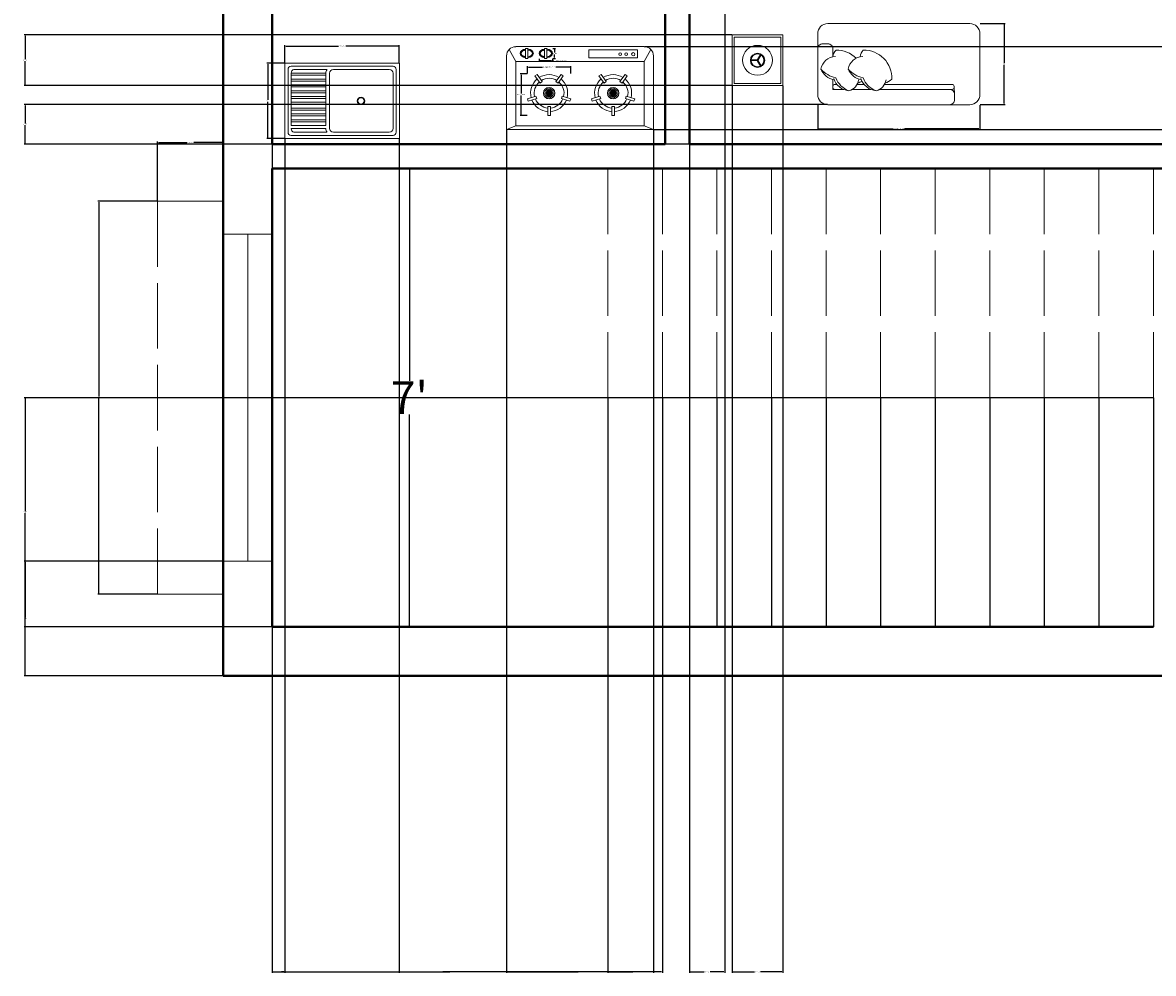
# Model space of a CAD drawing. Units: inches. Extents: x -22 to 362, y -469 to 42.
# Tile 1 of 6: x -22 to 186, y -469 to -295. Entities that reach past the tile are written whole.
import ezdxf

# ---------------------------------------------------------------- set-up
doc = ezdxf.new("R2010")
doc.units = ezdxf.units.IN
doc.header["$MEASUREMENT"] = 0
doc.linetypes.add('ACAD_ISO02W100', pattern=[15, 12, -3])
for name, color, linetype, lineweight in [('A-ANNO-DIMS', 2, 'Continuous', 18), ('A-EQPM', 8, 'Continuous', 18), ('A-FLOR-FIXT', 9, 'Continuous', 20), ('A-FLOR-STRS', 7, 'Continuous', 25), ('A-FLOR-STRS-OVHD', 7, 'ACAD_ISO02W100', 18), ('A-FURN', 8, 'Continuous', 18), ('A-GLAZ', 4, 'Continuous', 20), ('A-ROOF-OVHD', 8, 'ACAD_ISO02W100', 18), ('A-WALL', 7, 'Continuous', 40)]:
    doc.layers.add(name, color=color, linetype=linetype, lineweight=lineweight)
doc.styles.get("Standard").update_dxf_attribs({"font": 'arial.ttf'})
doc.dimstyles.get("Standard").update_dxf_attribs({"dimtxt": 0.18, "dimasz": 0.18, "dimexe": 0.18, "dimexo": 0.0625, "dimgap": 0.09, "dimtad": 0, "dimtih": 1, "dimtoh": 1, "dimdec": 0, "dimzin": 0, "dimdsep": 46, "dimlunit": 3, "dimtxsty": 'Standard', "dimcen": 0.09, "dimadec": 0, "dimazin": 0, "dimtfac": 1, "dimtdec": 0, "dimtofl": 0, "dimtmove": 0, "dimatfit": 3, "dimfxl": 1, "dimtolj": 1, "dimtzin": 0, "dimarcsym": 0})

# ---------------------------------------------------------------- blocks, each defined once
blk = doc.blocks.new('*D1')
at = {"layer": 'A-ANNO-DIMS', "color": 0, "lineweight": -2, "transparency": 16777216}
for p, q in [((49.07, -321.31), (48.96, -321.31)), ((49.14, -321.49), (49.14, -360.22)), ((49.14, -405.13), (49.14, -366.4)), ((49.2, -405.31), (49.32, -405.31))]:
    blk.add_line(p, q, dxfattribs=at)
at = {"layer": 'A-ANNO-DIMS', "color": 0, "transparency": 16777216}
for points in [[(49.11, -321.49), (49.17, -321.49), (49.14, -321.31)], [(49.11, -405.13), (49.17, -405.13), (49.14, -405.31)]]:
    blk.add_solid(points, dxfattribs=at)
at = {"layer": 'Defpoints', "color": 0, "transparency": 16777216}
for p in [(49.14, -321.31), (49.14, -405.31), (49.14, -405.31)]:
    blk.add_point(p, dxfattribs=at)
at = {"layer": 'A-ANNO-DIMS', "color": 0, "transparency": 16777216, "insert": (49.14, -363.31), "char_height": 6, "attachment_point": 5}
blk.add_mtext("\\A1;7'", dxfattribs=at)
blk = doc.blocks.new('DAY BED1')
at = {"color": 0}
blk.add_line((0.3, 0.25), (0.225, 0.255), dxfattribs=at)
blk.add_lwpolyline([(-0.3, 0, -0.414214), (-0.4, 0.1), (-0.4, 0.1, 0.317837), (-0.4, 0.1, -0.414214), (-0.4, 0.1), (-0.4, 0.1, 1.186185), (-0.4, 0.1, -0.414214), (-0.4, 0.1), (-0.4, 1.5, -0.414214), (-0.3, 1.6), (0.3, 1.6, -0.414214), (0.4, 1.5), (0.4, 0.1, -0.414214), (0.3, 0)], format="xyb", close=True, dxfattribs=at)
for points in [[(-0.073, 1.45), (-0.15, 1.45, -0.414214), (-0.2, 1.5), (-0.2, 1.55, -0.414214), (-0.15, 1.6)], [(-0.076, 1.425, -0.356772), (0.05, 1.568, -0.249542), (0.154, 1.438, 9.61688)], [(0.05, 1.568, -0.14773), (0.136, 1.422, -0.213343), (0.262, 1.293, -0.178662)], [(-0.073, 1.45, 0.165541), (-0.139, 1.419, 0.200231), (-0.058, 1.221, 0.121523)], [(0.25, 1.345), (0.25, 1.45), (0.152, 1.45, -0.414214)], [(0.2, 1.412), (0.2, 1.43, -0.414214), (0.22, 1.45), (0.23, 1.45, -0.414214), (0.25, 1.43)], [(0.143, 1.442, -0.306663), (0.262, 1.293, -0.30633), (0.154, 1.196, 0.872847)], [(0.25, 1.43), (0.25, 1.345, -0.414214)], [(-0.076, 1.156, -0.356772), (0.05, 1.299, -0.249542), (0.154, 1.169, 9.61688)], [(0.05, 1.299, -0.14773), (0.136, 1.153, -0.213343), (0.262, 1.024, -0.178662)], [(0.25, 1.262), (0.25, 1.075, -0.414214)], [(-0.073, 1.181, 0.165541), (-0.139, 1.15, 0.425989), (0.148, 0.869, 0.121523), (0.187, 0.936, -7.115464)], [(0.143, 1.173, -0.306663), (0.262, 1.024, -0.30633), (0.154, 0.926, 0.872847)], [(0.168, 1.163, 0.071865), (0.187, 1.205, -7.115464)], [(0.2, 1.142), (0.2, 1.211, -0.414214)], [(0.25, 0.992), (0.25, 0.275, -0.414214), (0.23, 0.255), (0.22, 0.255, -0.414214), (0.2, 0.275), (0.2, 0.942, -0.414214)], [(0.25, 0.377), (0.25, 0.3, 0.414214), (0.3, 0.25), (0.35, 0.25, 0.414214), (0.4, 0.3)]]:
    blk.add_lwpolyline(points, format="xyb", dxfattribs=at)
for points in [[(0.25, 1.075), (0.25, 1.262)], [(0.25, 0.377), (0.25, 0.992)]]:
    blk.add_lwpolyline(points, dxfattribs=at)
blk = doc.blocks.new('М12 540х820')
for p, q in [((0, 540), (-820, 540)), ((-820, 540), (-820, 0)), ((-797.5, 495), (-797.5, 45)), ((-45, 517.5), (-775, 517.5)), ((-347.5, 495), (-748, 495)), ((-301.7, 495), (-64.8, 495)), ((-22.5, 45), (-22.5, 495)), ((0, 0), (0, 540)), ((-775, 468), (-775, 72)), ((-320.5, 468), (-320.5, 72)), ((-293.7, 468), (-293.7, 472.5)), ((-293.7, 468), (-45, 468)), ((-293.7, 446.6), (-45, 446.6)), ((-293.7, 419.6), (-293.7, 446.6)), ((-293.7, 419.6), (-45, 419.6)), ((-45, 469.5), (-45, 468)), ((-45, 419.6), (-45, 446.6)), ((-293.7, 405), (-45, 405)), ((-293.7, 378), (-293.7, 405)), ((-293.7, 378), (-45, 378)), ((-293.7, 336.4), (-293.7, 363.4)), ((-293.7, 363.4), (-45, 363.4)), ((-293.7, 336.4), (-45, 336.4)), ((-45, 378), (-45, 405)), ((-45, 336.4), (-45, 363.4)), ((-293.7, 294.7), (-293.7, 321.7)), ((-293.7, 321.7), (-45, 321.7)), ((-293.7, 294.7), (-45, 294.7)), ((-293.7, 253.1), (-293.7, 280.1)), ((-293.7, 280.1), (-45, 280.1)), ((-293.7, 253.1), (-45, 253.1)), ((-45, 294.7), (-45, 321.7)), ((-45, 253.1), (-45, 280.1)), ((-293.7, 211.5), (-293.7, 238.5)), ((-293.7, 238.5), (-45, 238.5)), ((-293.7, 211.5), (-45, 211.5)), ((-293.7, 169.9), (-293.7, 196.9)), ((-293.7, 196.9), (-45, 196.9)), ((-293.7, 169.9), (-45, 169.9)), ((-45, 211.5), (-45, 238.5)), ((-45, 169.9), (-45, 196.9)), ((-293.7, 128.2), (-293.7, 155.2)), ((-293.7, 155.2), (-45, 155.2)), ((-293.7, 128.2), (-45, 128.2)), ((-293.7, 113.6), (-45, 113.6)), ((-293.7, 86.6), (-293.7, 113.6)), ((-293.7, 86.6), (-45, 86.6)), ((-45, 128.2), (-45, 155.2)), ((-45, 86.6), (-45, 113.6)), ((-820, 0), (0, 0)), ((-775, 22.5), (-45, 22.5)), ((-748, 45), (-347.5, 45)), ((-301.7, 45), (-64.8, 45)), ((-293.7, 72), (-45, 72)), ((-45, 70.5), (-45, 72))]:
    blk.add_line(p, q)
at = {"ltscale": 0.06}
for p, q in [((-820, 0), (-820, 540)), ((-820, 540), (0, 540)), ((0, 540), (0, 536.9)), ((0, 536.9), (0, 0)), ((-293.7, 446.6), (-45, 446.6)), ((-293.7, 405), (-293.7, 446.6)), ((-45, 446.6), (-45, 419.6)), ((-45, 419.6), (-45, 378)), ((-293.7, 363.4), (-293.7, 405)), ((-293.7, 321.7), (-293.7, 363.4)), ((-45, 378), (-45, 336.4)), ((-45, 336.4), (-45, 294.7)), ((-293.7, 280.1), (-293.7, 321.7)), ((-293.7, 238.5), (-293.7, 280.1)), ((-45, 294.7), (-45, 253.1)), ((-45, 253.1), (-45, 211.5)), ((-293.7, 196.9), (-293.7, 238.5)), ((-293.7, 155.2), (-293.7, 196.9)), ((-45, 211.5), (-45, 169.9)), ((-45, 169.9), (-45, 128.2)), ((-293.7, 113.6), (-293.7, 155.2)), ((-293.7, 72), (-293.7, 113.6)), ((-45, 128.2), (-45, 86.6)), ((-45, 86.6), (-45, 72)), ((0, 0), (-820, 0)), ((-45, 72), (-293.7, 72))]:
    blk.add_line(p, q, dxfattribs=at)
at = {"extrusion": (0, 0, -1)}
for centre, major_axis, start_param, end_param in [((-775, 495), (-15.9, 15.9), -0.785398, 0.785398), ((-775, 495), (-15.9, 15.9), -0.785398, 0.785398), ((-748, 468), (-19.1, -19.1), 0.785398, 2.356194), ((-748, 468), (-19.1, -19.1), 0.785398, 2.356194), ((-347.5, 468), (-19.1, 19.1), 0.785398, 2.356194), ((-347.5, 468), (-19.1, 19.1), 0.785398, 2.356194), ((-343.2, 468), (-35, 35), 1.779263, 2.356194), ((-343.2, 468), (-35, 35), 1.779263, 2.356192), ((-72.3, 468.8), (-19.3, 19.3), 1.0328, 2.38382), ((-72.3, 468.8), (-19.3, 19.3), 1.0328, 1.064673), ((-72.3, 468.8), (-19.3, 19.3), 1.064673, 2.328569), ((-45, 495), (-15.9, -15.9), 2.356194, 3.926991), ((-45, 495), (-15.9, -15.9), 2.356194, 3.926991), ((-343.2, 468), (-35, 35), 2.356192, 2.356194), ((-72.3, 468.8), (-19.3, 19.3), 2.328569, 2.38382), ((-545.5, 270), (-19.1, -19.1), 3.926991, 10.210176), ((-545.5, 270), (-19.1, -19.1), 3.926991, 10.210176), ((-545.5, 270), (-15.9, -15.9), 3.926991, 10.210176), ((-545.5, 270), (-15.9, -15.9), 3.926991, 10.210176), ((-775, 45), (-15.9, -15.9), 5.497787, 7.068583), ((-775, 45), (-15.9, -15.9), 5.497787, 7.068583), ((-748, 72), (-19.1, 19.1), 3.926991, 5.497787), ((-748, 72), (-19.1, 19.1), 3.926991, 5.497787), ((-347.5, 72), (-19.1, -19.1), 3.926991, 5.497787), ((-347.5, 72), (-19.1, -19.1), 3.926991, 5.497787), ((-343.2, 72), (-35, -35), 3.926991, 4.503922), ((-343.2, 72), (-35, -35), 3.926991, 4.503922), ((-72.3, 71.2), (-19.3, -19.3), 3.899365, 5.250385), ((-72.3, 71.2), (-19.3, -19.3), 5.218512, 5.250385), ((-72.3, 71.2), (-19.3, -19.3), 3.954617, 5.218512), ((-72.3, 71.2), (-19.3, -19.3), 3.899365, 3.954617), ((-45, 45), (-15.9, 15.9), 2.356194, 3.926991), ((-45, 45), (-15.9, 15.9), 2.356194, 3.926991)]:
    blk.add_ellipse(centre, major_axis=major_axis, ratio=1, start_param=start_param, end_param=end_param, dxfattribs=at)
blk = doc.blocks.new('WIN-60-WALL9')
for p, q in [((0, 9), (60, 9)), ((0, 0), (0, 9)), ((60, 9), (60, 0)), ((0, 4.5), (60, 4.5)), ((60, 0), (0, 0))]:
    blk.add_line(p, q)
blk = doc.blocks.new('WINDOW-SHADE-72')
for p, q in [((12, 72), (0, 72)), ((12, 0), (12, 72)), ((0, 0), (12, 0))]:
    blk.add_line(p, q)
blk = doc.blocks.new('COOKTOP-BURNER')
for p, q in [((-2.59, 3.18), (-2.22, 3.45)), ((-1.63, 1.85), (-2.59, 3.18)), ((-2.22, 3.45), (-1.26, 2.12)), ((-1.26, 2.12), (-1.63, 1.85)), ((1.26, 2.12), (2.22, 3.45)), ((1.63, 1.85), (1.26, 2.12)), ((2.59, 3.18), (1.63, 1.85)), ((2.22, 3.45), (2.59, 3.18)), ((0, 0), (-1.04, 0)), ((0, 0), (-0.99, 0.32)), ((0, 0), (-0.99, -0.32)), ((0, 0), (-0.84, 0.61)), ((0, 0), (-0.84, -0.61)), ((0, 0), (-0.61, 0.84)), ((0, 0), (-0.61, -0.84)), ((0, 0), (-0.32, 0.99)), ((0, 0), (-0.32, -0.99)), ((0, 0), (0, 1.04)), ((0, 0), (0.32, 0.99)), ((0, 0), (0.61, 0.84)), ((0, 0), (0.84, 0.61)), ((0, 0), (0.99, 0.32)), ((0, 0), (1.04, 0)), ((0, 0), (0.99, -0.32)), ((0, 0), (0.84, -0.61)), ((0, 0), (0.61, -0.84)), ((0, 0), (0.32, -0.99)), ((0, 0), (0, -1.04)), ((-3.96, -1.05), (-2.41, -0.54)), ((-3.82, -1.48), (-3.96, -1.05)), ((-2.26, -0.98), (-3.82, -1.48)), ((-2.41, -0.54), (-2.26, -0.98)), ((2.26, -0.98), (2.41, -0.54)), ((3.82, -1.48), (2.26, -0.98)), ((2.41, -0.54), (3.96, -1.05)), ((3.96, -1.05), (3.82, -1.48)), ((-0.23, -2.46), (0.23, -2.46)), ((-0.23, -4.09), (-0.23, -2.46)), ((0.23, -4.09), (-0.23, -4.09)), ((0.23, -2.46), (0.23, -4.09))]:
    blk.add_line(p, q)
blk.add_circle((0, 0), 1.04)
for radius, start, end in [(3.4, 129.8765, 194.1235), (3.4, 57.8765, 122.1235), (2.73, 58.8365, 121.1635), (3.4, 345.8765, 50.1235), (2.73, 130.8365, 193.1635), (2.73, 346.8365, 49.1635), (3.4, 201.8765, 266.1235), (2.73, 202.8365, 265.1635), (2.73, 274.8365, 337.1635), (3.4, 273.8765, 338.1235)]:
    blk.add_arc((0, 0), radius, start, end)
blk = doc.blocks.new('COOKTOP-CONTROL')
for p, q in [((0, 0), (0, 1.86)), ((0, 1.86), (0.44, 1.86)), ((0.44, 0), (0, 0)), ((0.44, 1.86), (0.44, 0))]:
    blk.add_line(p, q)
for major_axis, start_param, end_param in [((1.21, 0), 1.774361, 4.508825), ((-1.21, 0), 1.73081, 4.552375)]:
    blk.add_ellipse((0.24, 0.94), major_axis=major_axis, ratio=0.671641, start_param=start_param, end_param=end_param)
for points, knots in [([(0, 1.56), (-0.06, 1.55), (-0.12, 1.54), (-0.24, 1.51), (-0.31, 1.48), (-0.44, 1.42), (-0.5, 1.39), (-0.59, 1.32), (-0.64, 1.28), (-0.71, 1.2), (-0.73, 1.15), (-0.77, 1.07), (-0.78, 1.03), (-0.8, 0.95), (-0.79, 0.91), (-0.78, 0.83), (-0.76, 0.79), (-0.72, 0.7), (-0.69, 0.66), (-0.61, 0.58), (-0.57, 0.54), (-0.46, 0.47), (-0.4, 0.44), (-0.27, 0.39), (-0.2, 0.36), (-0.09, 0.33), (-0.04, 0.32), (0, 0.32)], [8.079302, 8.079302, 8.079302, 8.079302, 8.245651, 8.245651, 8.463703, 8.463703, 8.681755, 8.681755, 8.899807, 8.899807, 9.117859, 9.117859, 9.33591, 9.33591, 9.553962, 9.553962, 9.772014, 9.772014, 9.990066, 9.990066, 10.208118, 10.208118, 10.426169, 10.426169, 10.644221, 10.644221, 10.770253, 10.770253, 10.770253, 10.770253]), ([(0.44, 0.31), (0.48, 0.32), (0.53, 0.32), (0.64, 0.35), (0.72, 0.37), (0.85, 0.42), (0.91, 0.45), (1.02, 0.52), (1.07, 0.56), (1.15, 0.64), (1.19, 0.68), (1.24, 0.76), (1.26, 0.8), (1.28, 0.87), (1.28, 0.91), (1.28, 0.94), (1.28, 0.98), (1.27, 1.02), (1.25, 1.1), (1.23, 1.15), (1.17, 1.23), (1.13, 1.27), (1.05, 1.35), (0.99, 1.38), (0.88, 1.45), (0.81, 1.48), (0.68, 1.52), (0.6, 1.54), (0.5, 1.56), (0.47, 1.57), (0.44, 1.57)], [4.889299, 4.889299, 4.889299, 4.889299, 5.015191, 5.015191, 5.233243, 5.233243, 5.451295, 5.451295, 5.669347, 5.669347, 5.887399, 5.887399, 6.10545, 6.10545, 6.283185, 6.283185, 6.283185, 6.501237, 6.501237, 6.719289, 6.719289, 6.937341, 6.937341, 7.155392, 7.155392, 7.373444, 7.373444, 7.591496, 7.591496, 7.677072, 7.677072, 7.677072, 7.677072])]:
    blk.add_open_spline(points, degree=3, knots=knots)
blk = doc.blocks.new('*D16')
at = {"layer": 'A-ANNO-DIMS', "color": 0, "lineweight": -2, "transparency": 16777216}
for p, q in [((2.95, -327.31), (-7.97, -327.31)), ((-7.79, -327.49), (-7.79, -363.12)), ((-7.79, -399.13), (-7.79, -363.49)), ((2.95, -399.31), (-7.97, -399.31))]:
    blk.add_line(p, q, dxfattribs=at)
at = {"layer": 'A-ANNO-DIMS', "color": 0, "transparency": 16777216}
for points in [[(-7.82, -327.49), (-7.76, -327.49), (-7.79, -327.31)], [(-7.82, -399.13), (-7.76, -399.13), (-7.79, -399.31)]]:
    blk.add_solid(points, dxfattribs=at)
at = {"layer": 'Defpoints', "color": 0, "transparency": 16777216}
for p in [(3.01, -327.31), (-7.79, -399.31), (3.01, -399.31)]:
    blk.add_point(p, dxfattribs=at)
at = {"layer": 'A-ANNO-DIMS', "color": 0, "transparency": 16777216, "insert": (-7.79, -363.31), "char_height": 0.18, "attachment_point": 5}
blk.add_mtext('\\A1;SHADE 6\'-0" TYP.', dxfattribs=at)
blk = doc.blocks.new('*D17')
at = {"layer": 'A-ANNO-DIMS', "color": 0, "lineweight": -2, "transparency": 16777216}
for p, q in [((3.01, -327.24), (3.01, -316.33)), ((3.19, -316.51), (8.38, -316.51)), ((14.83, -316.51), (9.64, -316.51)), ((15.01, -327.24), (15.01, -316.33))]:
    blk.add_line(p, q, dxfattribs=at)
at = {"layer": 'A-ANNO-DIMS', "color": 0, "transparency": 16777216}
for points in [[(3.19, -316.48), (3.19, -316.54), (3.01, -316.51)], [(14.83, -316.48), (14.83, -316.54), (15.01, -316.51)]]:
    blk.add_solid(points, dxfattribs=at)
at = {"layer": 'Defpoints', "color": 0, "transparency": 16777216}
for p in [(3.01, -316.51), (3.01, -327.31), (15.01, -327.31)]:
    blk.add_point(p, dxfattribs=at)
at = {"layer": 'A-ANNO-DIMS', "color": 0, "transparency": 16777216, "insert": (9.01, -316.51), "char_height": 0.18, "attachment_point": 5}
blk.add_mtext('\\A1;1\'-0" TYP.', dxfattribs=at)
blk = doc.blocks.new('*D24')
at = {"layer": 'A-ANNO-DIMS', "color": 0, "lineweight": -2, "transparency": 16777216}
for p, q in [((70.79, -303.85), (70.79, -302.55)), ((78.72, -303.85), (78.72, -302.55)), ((70.97, -302.73), (73.56, -302.73)), ((78.54, -302.73), (75.96, -302.73))]:
    blk.add_line(p, q, dxfattribs=at)
at = {"layer": 'A-ANNO-DIMS', "color": 0, "transparency": 16777216}
for points in [[(70.97, -302.7), (70.97, -302.76), (70.79, -302.73)], [(78.54, -302.7), (78.54, -302.76), (78.72, -302.73)]]:
    blk.add_solid(points, dxfattribs=at)
at = {"layer": 'Defpoints', "color": 0, "transparency": 16777216}
for p in [(70.79, -303.92), (78.72, -302.73), (78.72, -303.92)]:
    blk.add_point(p, dxfattribs=at)
at = {"layer": 'A-ANNO-DIMS', "color": 0, "transparency": 16777216, "insert": (74.76, -302.73), "char_height": 0.18, "attachment_point": 5}
blk.add_mtext('\\A1;BURNER 0\'-8" TYP.', dxfattribs=at)
blk = doc.blocks.new('*D25')
at = {"layer": 'A-ANNO-DIMS', "color": 0, "lineweight": -2, "transparency": 16777216}
for p, q in [((70.73, -303.92), (69.43, -303.92)), ((69.61, -304.1), (69.61, -307.57)), ((69.61, -311.4), (69.61, -307.93)), ((70.73, -311.58), (69.43, -311.58))]:
    blk.add_line(p, q, dxfattribs=at)
at = {"layer": 'A-ANNO-DIMS', "color": 0, "transparency": 16777216}
for points in [[(69.58, -304.1), (69.64, -304.1), (69.61, -303.92)], [(69.58, -311.4), (69.64, -311.4), (69.61, -311.58)]]:
    blk.add_solid(points, dxfattribs=at)
at = {"layer": 'Defpoints', "color": 0, "transparency": 16777216}
for p in [(69.61, -303.92), (70.79, -303.92), (70.79, -311.58)]:
    blk.add_point(p, dxfattribs=at)
at = {"layer": 'A-ANNO-DIMS', "color": 0, "transparency": 16777216, "insert": (69.61, -307.75), "char_height": 0.18, "attachment_point": 5}
blk.add_mtext('\\A1;0\'-7 1/2" TYP.', dxfattribs=at)
blk = doc.blocks.new('*D26')
at = {"layer": 'A-ANNO-DIMS', "color": 0, "lineweight": -2, "transparency": 16777216}
for p, q in [((72.96, -301.19), (72.96, -301.67)), ((73.14, -301.49), (75.19, -301.49)), ((75.37, -301.19), (75.37, -301.67)), ((75.37, -301.49), (75.55, -301.49))]:
    blk.add_line(p, q, dxfattribs=at)
at = {"layer": 'A-ANNO-DIMS', "color": 0, "transparency": 16777216}
for points in [[(73.14, -301.46), (73.14, -301.52), (72.96, -301.49)], [(75.19, -301.46), (75.19, -301.52), (75.37, -301.49)]]:
    blk.add_solid(points, dxfattribs=at)
at = {"layer": 'Defpoints', "color": 0, "transparency": 16777216}
for p in [(72.96, -301.13), (75.37, -301.13), (75.37, -301.49)]:
    blk.add_point(p, dxfattribs=at)
at = {"layer": 'A-ANNO-DIMS', "color": 0, "transparency": 16777216, "insert": (76.79, -301.49), "char_height": 0.18, "attachment_point": 5}
blk.add_mtext('\\A1;KNOB 0\'-2 1/2" TYP.', dxfattribs=at)
blk = doc.blocks.new('*D27')
at = {"layer": 'A-ANNO-DIMS', "color": 0, "lineweight": -2, "transparency": 16777216}
for p, q in [((75.44, -299.27), (75.92, -299.27)), ((75.74, -299.45), (75.74, -300.02)), ((75.74, -300.95), (75.74, -300.38)), ((75.44, -301.13), (75.92, -301.13))]:
    blk.add_line(p, q, dxfattribs=at)
at = {"layer": 'A-ANNO-DIMS', "color": 0, "transparency": 16777216}
for points in [[(75.71, -299.45), (75.77, -299.45), (75.74, -299.27)], [(75.71, -300.95), (75.77, -300.95), (75.74, -301.13)]]:
    blk.add_solid(points, dxfattribs=at)
at = {"layer": 'Defpoints', "color": 0, "transparency": 16777216}
for p in [(75.37, -299.27), (75.74, -299.27), (75.37, -301.13)]:
    blk.add_point(p, dxfattribs=at)
at = {"layer": 'A-ANNO-DIMS', "color": 0, "transparency": 16777216, "insert": (75.74, -300.2), "char_height": 0.18, "attachment_point": 5}
blk.add_mtext('\\A1;0\'-2" TYP.', dxfattribs=at)
blk = doc.blocks.new('*D28')
at = {"layer": 'A-ANNO-DIMS', "color": 0, "lineweight": -2, "transparency": 16777216}
for p, q in [((123.98, -309.66), (123.98, -314.23)), ((153.72, -309.66), (153.72, -314.23)), ((124.16, -314.05), (137.79, -314.05)), ((153.54, -314.05), (139.91, -314.05))]:
    blk.add_line(p, q, dxfattribs=at)
at = {"layer": 'A-ANNO-DIMS', "color": 0, "transparency": 16777216}
for points in [[(124.16, -314.02), (124.16, -314.08), (123.98, -314.05)], [(153.54, -314.02), (153.54, -314.08), (153.72, -314.05)]]:
    blk.add_solid(points, dxfattribs=at)
at = {"layer": 'Defpoints', "color": 0, "transparency": 16777216}
for p in [(123.98, -309.59), (153.72, -309.59), (123.98, -314.05)]:
    blk.add_point(p, dxfattribs=at)
at = {"layer": 'A-ANNO-DIMS', "color": 0, "transparency": 16777216, "insert": (138.85, -314.05), "char_height": 0.18, "attachment_point": 5}
blk.add_mtext('\\A1;SETTEE 2\'-5 1/2"', dxfattribs=at)
blk = doc.blocks.new('*D29')
at = {"layer": 'A-ANNO-DIMS', "color": 0, "lineweight": -2, "transparency": 16777216}
for p, q in [((153.78, -294.73), (158.36, -294.73)), ((158.18, -294.91), (158.18, -301.98)), ((158.18, -309.41), (158.18, -302.34)), ((153.78, -309.59), (158.36, -309.59))]:
    blk.add_line(p, q, dxfattribs=at)
at = {"layer": 'A-ANNO-DIMS', "color": 0, "transparency": 16777216}
for points in [[(158.15, -294.91), (158.21, -294.91), (158.18, -294.73)], [(158.15, -309.41), (158.21, -309.41), (158.18, -309.59)]]:
    blk.add_solid(points, dxfattribs=at)
at = {"layer": 'Defpoints', "color": 0, "transparency": 16777216}
for p in [(153.72, -294.73), (153.72, -309.59), (158.18, -309.59)]:
    blk.add_point(p, dxfattribs=at)
at = {"layer": 'A-ANNO-DIMS', "color": 0, "transparency": 16777216, "insert": (158.18, -302.16), "char_height": 0.18, "attachment_point": 5}
blk.add_mtext('\\A1;1\'-3"', dxfattribs=at)
blk = doc.blocks.new('*D30')
at = {"layer": 'A-ANNO-DIMS', "color": 0, "lineweight": -2, "transparency": 16777216}
for p, q in [((26.33, -301.93), (26.33, -298.66)), ((26.51, -298.84), (36.16, -298.84)), ((47.12, -298.84), (37.47, -298.84)), ((47.3, -301.93), (47.3, -298.66))]:
    blk.add_line(p, q, dxfattribs=at)
at = {"layer": 'A-ANNO-DIMS', "color": 0, "transparency": 16777216}
for points in [[(26.51, -298.81), (26.51, -298.87), (26.33, -298.84)], [(47.12, -298.81), (47.12, -298.87), (47.3, -298.84)]]:
    blk.add_solid(points, dxfattribs=at)
at = {"layer": 'Defpoints', "color": 0, "transparency": 16777216}
for p in [(26.33, -298.84), (26.33, -301.99), (47.3, -301.99)]:
    blk.add_point(p, dxfattribs=at)
at = {"layer": 'A-ANNO-DIMS', "color": 0, "transparency": 16777216, "insert": (36.81, -298.84), "char_height": 0.18, "attachment_point": 5}
blk.add_mtext('\\A1;SINK 1\'-9"', dxfattribs=at)
blk = doc.blocks.new('*D31')
at = {"layer": 'A-ANNO-DIMS', "color": 0, "lineweight": -2, "transparency": 16777216}
for p, q in [((26.26, -301.99), (23, -301.99)), ((23.18, -302.17), (23.18, -308.72)), ((23.18, -315.62), (23.18, -309.08)), ((26.26, -315.8), (23, -315.8))]:
    blk.add_line(p, q, dxfattribs=at)
at = {"layer": 'A-ANNO-DIMS', "color": 0, "transparency": 16777216}
for points in [[(23.15, -302.17), (23.21, -302.17), (23.18, -301.99)], [(23.15, -315.62), (23.21, -315.62), (23.18, -315.8)]]:
    blk.add_solid(points, dxfattribs=at)
at = {"layer": 'Defpoints', "color": 0, "transparency": 16777216}
for p in [(26.33, -301.99), (23.18, -315.8), (26.33, -315.8)]:
    blk.add_point(p, dxfattribs=at)
at = {"layer": 'A-ANNO-DIMS', "color": 0, "transparency": 16777216, "insert": (23.18, -308.9), "char_height": 0.18, "attachment_point": 5}
blk.add_mtext('\\A1;1\'-2"', dxfattribs=at)
blk = doc.blocks.new('*D37')
at = {"layer": 'A-ANNO-DIMS', "color": 0, "lineweight": -2, "transparency": 16777216}
for p, q in [((14.95, -393.31), (-21.45, -393.31)), ((-21.27, -393.49), (-21.27, -403.62)), ((-21.27, -414.13), (-21.27, -403.99)), ((14.95, -414.31), (-21.45, -414.31))]:
    blk.add_line(p, q, dxfattribs=at)
at = {"layer": 'A-ANNO-DIMS', "color": 0, "transparency": 16777216}
for points in [[(-21.3, -393.49), (-21.24, -393.49), (-21.27, -393.31)], [(-21.3, -414.13), (-21.24, -414.13), (-21.27, -414.31)]]:
    blk.add_solid(points, dxfattribs=at)
at = {"layer": 'Defpoints', "color": 0, "transparency": 16777216}
for p in [(15.01, -393.31), (-21.27, -414.31), (15.01, -414.31)]:
    blk.add_point(p, dxfattribs=at)
at = {"layer": 'A-ANNO-DIMS', "color": 0, "transparency": 16777216, "insert": (-21.27, -403.81), "char_height": 0.18, "attachment_point": 5}
blk.add_mtext('\\A1;1\'-9"', dxfattribs=at)
blk = doc.blocks.new('*D44')
at = {"layer": 'A-ANNO-DIMS', "color": 0, "lineweight": -2, "transparency": 16777216}
for p, q in [((24.01, -405.37), (24.01, -468.77)), ((85.51, -405.37), (85.51, -468.77)), ((24.19, -468.59), (54.22, -468.59)), ((85.33, -468.59), (55.3, -468.59))]:
    blk.add_line(p, q, dxfattribs=at)
at = {"layer": 'A-ANNO-DIMS', "color": 0, "transparency": 16777216}
for points in [[(24.19, -468.56), (24.19, -468.62), (24.01, -468.59)], [(85.33, -468.56), (85.33, -468.62), (85.51, -468.59)]]:
    blk.add_solid(points, dxfattribs=at)
at = {"layer": 'Defpoints', "color": 0, "transparency": 16777216}
for p in [(24.01, -405.31), (85.51, -405.31), (85.51, -468.59)]:
    blk.add_point(p, dxfattribs=at)
at = {"layer": 'A-ANNO-DIMS', "color": 0, "transparency": 16777216, "insert": (54.76, -468.59), "char_height": 0.18, "attachment_point": 5}
blk.add_mtext('\\A1;5\'-1 1/2"', dxfattribs=at)
blk = doc.blocks.new('*D45')
at = {"layer": 'A-ANNO-DIMS', "color": 0, "lineweight": -2, "transparency": 16777216}
for p, q in [((85.51, -405.37), (85.51, -468.77)), ((95.51, -405.37), (95.51, -468.77)), ((85.69, -468.59), (90.11, -468.59)), ((95.33, -468.59), (90.91, -468.59))]:
    blk.add_line(p, q, dxfattribs=at)
at = {"layer": 'A-ANNO-DIMS', "color": 0, "transparency": 16777216}
for points in [[(85.69, -468.56), (85.69, -468.62), (85.51, -468.59)], [(95.33, -468.56), (95.33, -468.62), (95.51, -468.59)]]:
    blk.add_solid(points, dxfattribs=at)
at = {"layer": 'Defpoints', "color": 0, "transparency": 16777216}
for p in [(85.51, -405.31), (95.51, -405.31), (95.51, -468.59)]:
    blk.add_point(p, dxfattribs=at)
at = {"layer": 'A-ANNO-DIMS', "color": 0, "transparency": 16777216, "insert": (90.51, -468.59), "char_height": 0.18, "attachment_point": 5}
blk.add_mtext('\\A1;0\'-10"', dxfattribs=at)
blk = doc.blocks.new('*D46')
at = {"layer": 'A-ANNO-DIMS', "color": 0, "lineweight": -2, "transparency": 16777216}
for p, q in [((85.45, -363.31), (-21.45, -363.31)), ((-21.27, -363.49), (-21.27, -384.12)), ((-21.27, -405.13), (-21.27, -384.49)), ((85.45, -405.31), (-21.45, -405.31))]:
    blk.add_line(p, q, dxfattribs=at)
at = {"layer": 'A-ANNO-DIMS', "color": 0, "transparency": 16777216}
for points in [[(-21.3, -363.49), (-21.24, -363.49), (-21.27, -363.31)], [(-21.3, -405.13), (-21.24, -405.13), (-21.27, -405.31)]]:
    blk.add_solid(points, dxfattribs=at)
at = {"layer": 'Defpoints', "color": 0, "transparency": 16777216}
for p in [(85.51, -363.31), (-21.27, -405.31), (85.51, -405.31)]:
    blk.add_point(p, dxfattribs=at)
at = {"layer": 'A-ANNO-DIMS', "color": 0, "transparency": 16777216, "insert": (-21.27, -384.31), "char_height": 0.18, "attachment_point": 5}
blk.add_mtext('\\A1;3\'-6"', dxfattribs=at)
blk = doc.blocks.new('*D52')
at = {"layer": 'A-ANNO-DIMS', "color": 0, "lineweight": -2, "transparency": 16777216}
for p, q in [((106.94, -292.58), (106.94, -468.77)), ((100.51, -316.87), (100.51, -468.77)), ((100.69, -468.59), (103.19, -468.59)), ((106.76, -468.59), (104.27, -468.59))]:
    blk.add_line(p, q, dxfattribs=at)
at = {"layer": 'A-ANNO-DIMS', "color": 0, "transparency": 16777216}
for points in [[(100.69, -468.56), (100.69, -468.62), (100.51, -468.59)], [(106.76, -468.56), (106.76, -468.62), (106.94, -468.59)]]:
    blk.add_solid(points, dxfattribs=at)
at = {"layer": 'Defpoints', "color": 0, "transparency": 16777216}
for p in [(106.94, -292.52), (100.51, -316.81), (106.94, -468.59)]:
    blk.add_point(p, dxfattribs=at)
at = {"layer": 'A-ANNO-DIMS', "color": 0, "transparency": 16777216, "insert": (103.73, -468.59), "char_height": 0.18, "attachment_point": 5}
blk.add_mtext('\\A1;0\'-6 1/2"', dxfattribs=at)
blk = doc.blocks.new('*D53')
at = {"layer": 'A-ANNO-DIMS', "color": 0, "lineweight": -2, "transparency": 16777216}
for p, q in [((125.78, -309.59), (-21.45, -309.59)), ((-21.27, -309.77), (-21.27, -313.02)), ((-21.27, -316.63), (-21.27, -313.38)), ((100.45, -316.81), (-21.45, -316.81))]:
    blk.add_line(p, q, dxfattribs=at)
at = {"layer": 'A-ANNO-DIMS', "color": 0, "transparency": 16777216}
for points in [[(-21.3, -309.77), (-21.24, -309.77), (-21.27, -309.59)], [(-21.3, -316.63), (-21.24, -316.63), (-21.27, -316.81)]]:
    blk.add_solid(points, dxfattribs=at)
at = {"layer": 'Defpoints', "color": 0, "transparency": 16777216}
for p in [(-21.27, -309.59), (125.84, -309.59), (100.51, -316.81)]:
    blk.add_point(p, dxfattribs=at)
at = {"layer": 'A-ANNO-DIMS', "color": 0, "transparency": 16777216, "insert": (-21.27, -313.2), "char_height": 0.18, "attachment_point": 5}
blk.add_mtext('\\A1;0\'-7"', dxfattribs=at)
blk = doc.blocks.new('*D58')
at = {"layer": 'A-ANNO-DIMS', "color": 0, "lineweight": -2, "transparency": 16777216}
for p, q in [((108.31, -306.17), (108.31, -468.77)), ((117.6, -306.17), (117.6, -468.77)), ((108.49, -468.59), (112.42, -468.59)), ((117.42, -468.59), (113.5, -468.59))]:
    blk.add_line(p, q, dxfattribs=at)
at = {"layer": 'A-ANNO-DIMS', "color": 0, "transparency": 16777216}
for points in [[(108.49, -468.56), (108.49, -468.62), (108.31, -468.59)], [(117.42, -468.56), (117.42, -468.62), (117.6, -468.59)]]:
    blk.add_solid(points, dxfattribs=at)
at = {"layer": 'Defpoints', "color": 0, "transparency": 16777216}
for p in [(108.31, -306.11), (117.6, -306.11), (117.6, -468.59)]:
    blk.add_point(p, dxfattribs=at)
at = {"layer": 'A-ANNO-DIMS', "color": 0, "transparency": 16777216, "insert": (112.96, -468.59), "char_height": 0.18, "attachment_point": 5}
blk.add_mtext('\\A1;0\'-9 1/2"', dxfattribs=at)
blk = doc.blocks.new('*D59')
at = {"layer": 'A-ANNO-DIMS', "color": 0, "lineweight": -2, "transparency": 16777216}
for p, q in [((108.25, -296.82), (-21.45, -296.82)), ((-21.27, -297), (-21.27, -301.28)), ((-21.27, -305.93), (-21.27, -301.64)), ((108.25, -306.11), (-21.45, -306.11))]:
    blk.add_line(p, q, dxfattribs=at)
at = {"layer": 'A-ANNO-DIMS', "color": 0, "transparency": 16777216}
for points in [[(-21.3, -297), (-21.24, -297), (-21.27, -296.82)], [(-21.3, -305.93), (-21.24, -305.93), (-21.27, -306.11)]]:
    blk.add_solid(points, dxfattribs=at)
at = {"layer": 'Defpoints', "color": 0, "transparency": 16777216}
for p in [(108.31, -296.82), (-21.27, -306.11), (108.31, -306.11)]:
    blk.add_point(p, dxfattribs=at)
at = {"layer": 'A-ANNO-DIMS', "color": 0, "transparency": 16777216, "insert": (-21.27, -301.46), "char_height": 0.18, "attachment_point": 5}
blk.add_mtext('\\A1;0\'-9 1/2"', dxfattribs=at)
blk = doc.blocks.new('*D60')
at = {"layer": 'A-ANNO-DIMS', "color": 0, "lineweight": -2, "transparency": 16777216}
for p, q in [((66.94, -314.19), (66.94, -468.77)), ((93.9, -314.19), (93.9, -468.77)), ((67.12, -468.59), (80.09, -468.59)), ((93.72, -468.59), (80.75, -468.59))]:
    blk.add_line(p, q, dxfattribs=at)
at = {"layer": 'A-ANNO-DIMS', "color": 0, "transparency": 16777216}
for points in [[(67.12, -468.56), (67.12, -468.62), (66.94, -468.59)], [(93.72, -468.56), (93.72, -468.62), (93.9, -468.59)]]:
    blk.add_solid(points, dxfattribs=at)
at = {"layer": 'Defpoints', "color": 0, "transparency": 16777216}
for p in [(66.94, -314.13), (93.9, -314.13), (93.9, -468.59)]:
    blk.add_point(p, dxfattribs=at)
at = {"layer": 'A-ANNO-DIMS', "color": 0, "transparency": 16777216, "insert": (80.42, -468.59), "char_height": 0.18, "attachment_point": 5}
blk.add_mtext('\\A1;2\'-3"', dxfattribs=at)
blk = doc.blocks.new('*D61')
at = {"layer": 'A-ANNO-DIMS', "color": 0, "lineweight": -2, "transparency": 16777216}
for p, q in [((92.28, -298.96), (350.97, -298.96)), ((350.79, -299.14), (350.79, -306.36)), ((350.79, -313.95), (350.79, -306.73)), ((93.96, -314.13), (350.97, -314.13))]:
    blk.add_line(p, q, dxfattribs=at)
at = {"layer": 'A-ANNO-DIMS', "color": 0, "transparency": 16777216}
for points in [[(350.76, -299.14), (350.82, -299.14), (350.79, -298.96)], [(350.76, -313.95), (350.82, -313.95), (350.79, -314.13)]]:
    blk.add_solid(points, dxfattribs=at)
at = {"layer": 'Defpoints', "color": 0, "transparency": 16777216}
for p in [(92.21, -298.96), (350.79, -298.96), (93.9, -314.13)]:
    blk.add_point(p, dxfattribs=at)
at = {"layer": 'A-ANNO-DIMS', "color": 0, "transparency": 16777216, "insert": (350.79, -306.55), "char_height": 0.18, "attachment_point": 5}
blk.add_mtext('\\A1;1\'-3"', dxfattribs=at)
blk = doc.blocks.new('*D62')
at = {"layer": 'A-ANNO-DIMS', "color": 0, "lineweight": -2, "transparency": 16777216}
for p, q in [((66.94, -314.19), (66.94, -468.77)), ((47.3, -315.87), (47.3, -468.77)), ((47.48, -468.59), (56.59, -468.59)), ((66.76, -468.59), (57.65, -468.59))]:
    blk.add_line(p, q, dxfattribs=at)
at = {"layer": 'A-ANNO-DIMS', "color": 0, "transparency": 16777216}
for points in [[(47.48, -468.56), (47.48, -468.62), (47.3, -468.59)], [(66.76, -468.56), (66.76, -468.62), (66.94, -468.59)]]:
    blk.add_solid(points, dxfattribs=at)
at = {"layer": 'Defpoints', "color": 0, "transparency": 16777216}
for p in [(66.94, -314.13), (47.3, -315.8), (66.94, -468.59)]:
    blk.add_point(p, dxfattribs=at)
at = {"layer": 'A-ANNO-DIMS', "color": 0, "transparency": 16777216, "insert": (57.12, -468.59), "char_height": 0.18, "attachment_point": 5}
blk.add_mtext('\\A1;1\'-7 1/2"', dxfattribs=at)
blk = doc.blocks.new('*D63')
at = {"layer": 'A-ANNO-DIMS', "color": 0, "lineweight": -2, "transparency": 16777216}
for p, q in [((24.01, -316.87), (24.01, -468.77)), ((26.33, -315.87), (26.33, -468.77)), ((24.19, -468.59), (24.63, -468.59)), ((26.15, -468.59), (25.71, -468.59))]:
    blk.add_line(p, q, dxfattribs=at)
at = {"layer": 'A-ANNO-DIMS', "color": 0, "transparency": 16777216}
for points in [[(24.19, -468.56), (24.19, -468.62), (24.01, -468.59)], [(26.15, -468.56), (26.15, -468.62), (26.33, -468.59)]]:
    blk.add_solid(points, dxfattribs=at)
at = {"layer": 'Defpoints', "color": 0, "transparency": 16777216}
for p in [(24.01, -316.81), (26.33, -315.8), (26.33, -468.59)]:
    blk.add_point(p, dxfattribs=at)
at = {"layer": 'A-ANNO-DIMS', "color": 0, "transparency": 16777216, "insert": (25.17, -468.59), "char_height": 0.18, "attachment_point": 5}
blk.add_mtext('\\A1;0\'-2 1/2"', dxfattribs=at)

msp = doc.modelspace()

# ---------------------------------------------------------------- linework, layer by layer
at = {"layer": 'A-EQPM'}
for p, q in [((68.63, -301.69), (67.44, -299.46)), ((92.21, -298.96), (68.63, -298.96)), ((82.01, -299.54), (90.93, -299.54)), ((82.01, -300.99), (82.01, -299.54)), ((90.93, -299.54), (90.93, -300.99)), ((92.21, -301.69), (93.41, -299.46)), ((66.94, -300.65), (66.94, -314.13)), ((68.63, -301.69), (68.63, -313.49)), ((92.21, -301.69), (68.63, -301.69)), ((90.93, -300.99), (82.01, -300.99)), ((92.21, -313.49), (92.21, -301.69)), ((93.9, -314.13), (93.9, -300.65)), ((68.63, -313.49), (66.94, -314.13)), ((66.94, -314.13), (93.9, -314.13)), ((68.63, -313.49), (92.21, -313.49)), ((92.21, -313.49), (93.9, -314.13))]:
    msp.add_line(p, q, dxfattribs=at)
for centre, radius in [((87.79, -300.34), 0.249), ((88.88, -300.34), 0.249), ((90.18, -300.34), 0.299)]:
    msp.add_circle(centre, radius, dxfattribs=at)
for centre, start, end in [((68.63, -300.65), 90, 180), ((92.21, -300.65), 0, 90)]:
    msp.add_arc(centre, 1.68, start, end, dxfattribs=at)
at = {"layer": 'A-FLOR-STRS'}
for p, q in [((185.51, -363.31), (85.51, -363.31)), ((85.51, -363.31), (85.51, -405.31)), ((95.51, -363.31), (95.51, -405.31)), ((105.51, -363.31), (105.51, -405.31)), ((115.51, -363.31), (115.51, -405.31)), ((125.51, -363.31), (125.51, -405.31)), ((135.51, -363.31), (135.51, -405.31)), ((145.51, -363.31), (145.51, -405.31)), ((155.51, -363.31), (155.51, -405.31)), ((165.51, -363.31), (165.51, -405.31)), ((175.51, -363.31), (175.51, -405.31)), ((185.51, -363.31), (185.51, -405.31))]:
    msp.add_line(p, q, dxfattribs=at)
at = {"layer": 'A-FLOR-STRS-OVHD'}
for p, q in [((85.51, -363.31), (85.51, -321.31)), ((95.51, -363.31), (95.51, -321.31)), ((105.51, -363.31), (105.51, -321.31)), ((115.51, -363.31), (115.51, -321.31)), ((125.51, -363.31), (125.51, -321.31)), ((135.51, -363.31), (135.51, -321.31)), ((145.51, -363.31), (145.51, -321.31)), ((155.51, -363.31), (155.51, -321.31)), ((165.51, -363.31), (165.51, -321.31)), ((175.51, -363.31), (175.51, -321.31)), ((185.51, -363.31), (185.51, -321.31))]:
    msp.add_line(p, q, dxfattribs=at)
at = {"layer": 'A-FURN'}
for p, q in [((112.91, -301.43), (113.56, -300.3)), ((113.01, -301.49), (113.66, -300.36)), ((112.96, -301.4), (111.65, -301.4)), ((112.96, -301.52), (111.65, -301.52)), ((112.91, -301.49), (113.56, -302.63)), ((113.01, -301.43), (113.66, -302.57))]:
    msp.add_line(p, q, dxfattribs=at)
at = {"layer": 'A-FURN', "ltscale": 0.03}
msp.add_lwpolyline([(117.6, -306.11), (117.6, -296.82), (108.31, -296.82), (108.31, -306.11)], close=True, dxfattribs=at)
at = {"layer": 'A-FURN'}
msp.add_lwpolyline([(117.23, -297.19), (117.23, -305.74), (108.68, -305.74), (108.68, -297.19)], close=True, dxfattribs=at)
for radius in [2.74, 1.31, 1.18]:
    msp.add_circle((112.96, -301.46), radius, dxfattribs=at)
at = {"layer": 'A-WALL'}
for p, q in [((15.01, 5.69), (15.01, -414.31)), ((24.01, -196.81), (24.01, -316.81)), ((96.01, -232.81), (96.01, -316.81)), ((100.51, -232.81), (100.51, -316.81)), ((24.01, -316.81), (96.01, -316.81)), ((100.51, -316.81), (269.51, -316.81)), ((24.01, -321.31), (269.51, -321.31)), ((24.01, -321.31), (24.01, -405.31)), ((24.01, -405.31), (185.51, -405.31)), ((15.01, -414.31), (314.51, -414.31))]:
    msp.add_line(p, q, dxfattribs=at)

# ---------------------------------------------------------------- block references
at = {"layer": 'A-EQPM'}
for name, p in [('COOKTOP-CONTROL', (70.43, -301.13)), ('COOKTOP-CONTROL', (73.92, -301.13)), ('COOKTOP-BURNER', (74.76, -307.49)), ('COOKTOP-BURNER', (86.49, -307.49))]:
    msp.add_blockref(name, p, dxfattribs=at)
at = {"layer": 'A-FLOR-FIXT', "xscale": 0.0255831846766497, "yscale": 0.0255831846766497, "zscale": 0.0255831846766497, "rotation": 180}
msp.add_blockref('М12 540х820', (26.33, -301.99), dxfattribs=at)
at = {"layer": 'A-FURN', "ltscale": 0.03, "xscale": -18.58445154306964, "yscale": 18.58445154306964, "zscale": 18.58445154306964, "rotation": 90}
msp.add_blockref('DAY BED1', (153.72, -302.16), dxfattribs=at)
at = {"layer": 'A-GLAZ', "rotation": 270}
msp.add_blockref('WIN-60-WALL9', (15.01, -333.31), dxfattribs=at)
at = {"layer": 'A-ROOF-OVHD', "rotation": 180}
msp.add_blockref('WINDOW-SHADE-72', (15.01, -327.31), dxfattribs=at)

# ---------------------------------------------------------------- dimensions: what is measured, and where the dimension line sits
at = {"layer": 'A-ANNO-DIMS'}
for base, p1, p2, picture, middle in [((106.94, -468.59), (100.51, -316.81), (106.94, -292.52), '*D52', (103.73, -468.59)), ((117.6, -468.59), (108.31, -306.11), (117.6, -306.11), '*D58', (112.96, -468.59)), ((66.94, -468.59), (47.3, -315.8), (66.94, -314.13), '*D62', (57.12, -468.59)), ((93.9, -468.59), (66.94, -314.13), (93.9, -314.13), '*D60', (80.42, -468.59)), ((26.33, -468.59), (24.01, -316.81), (26.33, -315.8), '*D63', (25.17, -468.59)), ((85.51, -468.59), (24.01, -405.31), (85.51, -405.31), '*D44', (54.76, -468.59)), ((95.51, -468.59), (85.51, -405.31), (95.51, -405.31), '*D45', (90.51, -468.59))]:
    dim = msp.add_linear_dim(base=base, p1=p1, p2=p2, dimstyle='Standard', override={"dimdec": 1, "dimlfac": 1, "dimrnd": 0, "dimzin": 1, "dimdsep": 46, "dimlunit": 4, "dimfrac": 2}, dxfattribs=at)
    dim.commit()
    dim.dimension.update_dxf_attribs({"geometry": picture, "text_midpoint": middle})
for base, p1, p2, angle, override, picture, middle in [((158.18, -309.59), (153.72, -294.73), (153.72, -309.59), 270, {"dimdec": 1, "dimlfac": 1, "dimrnd": 0, "dimzin": 1, "dimdsep": 46, "dimlunit": 4, "dimfrac": 2}, '*D29', (158.18, -302.16)), ((-21.27, -306.11), (108.31, -296.82), (108.31, -306.11), 90, {"dimdec": 1, "dimlfac": 1, "dimrnd": 0, "dimzin": 1, "dimdsep": 46, "dimlunit": 4, "dimfrac": 2}, '*D59', (-21.27, -301.46)), ((350.79, -298.96), (93.9, -314.13), (92.21, -298.96), 90, {"dimdec": 1, "dimlfac": 1, "dimrnd": 0, "dimzin": 1, "dimdsep": 46, "dimlunit": 4, "dimfrac": 2}, '*D61', (350.79, -306.55)), ((23.18, -315.8), (26.33, -301.99), (26.33, -315.8), 270, {"dimdec": 1, "dimlfac": 1, "dimrnd": 0, "dimzin": 1, "dimdsep": 46, "dimlunit": 4, "dimfrac": 2}, '*D31', (23.18, -308.9)), ((-21.27, -309.59), (100.51, -316.81), (125.84, -309.59), 90, {"dimdec": 1, "dimlfac": 1, "dimrnd": 0, "dimzin": 1, "dimdsep": 46, "dimlunit": 4, "dimfrac": 2}, '*D53', (-21.27, -313.2)), ((49.14, -405.31), (49.14, -321.31), (49.14, -405.31), 90, {"dimtxt": 6, "dimclrd": 0, "dimclre": 0, "dimclrt": 0}, '*D1', (49.14, -363.31)), ((-21.27, -405.31), (85.51, -363.31), (85.51, -405.31), 90, {"dimdec": 1, "dimlfac": 1, "dimrnd": 0, "dimzin": 1, "dimdsep": 46, "dimlunit": 4, "dimfrac": 2}, '*D46', (-21.27, -384.31)), ((-21.27, -414.31), (15.01, -393.31), (15.01, -414.31), 90, {"dimdec": 1, "dimlfac": 1, "dimrnd": 0, "dimzin": 1, "dimdsep": 46, "dimlunit": 4, "dimfrac": 2}, '*D37', (-21.27, -403.81))]:
    dim = msp.add_linear_dim(base=base, p1=p1, p2=p2, angle=angle, dimstyle='Standard', override=override, dxfattribs=at)
    dim.commit()
    dim.dimension.update_dxf_attribs({"geometry": picture, "text_midpoint": middle})
for base, p1, p2, angle, text, picture, middle in [((26.33, -298.84), (47.3, -301.99), (26.33, -301.99), 180, 'SINK <>', '*D30', (36.81, -298.84)), ((75.74, -299.27), (75.37, -301.13), (75.37, -299.27), 90, '<> TYP.', '*D27', (75.74, -300.2)), ((69.61, -303.92), (70.79, -311.58), (70.79, -303.92), 90, '<> TYP.', '*D25', (69.61, -307.75)), ((123.98, -314.05), (153.72, -309.59), (123.98, -309.59), 180, 'SETTEE <>', '*D28', (138.85, -314.05)), ((3.01, -316.51), (15.01, -327.31), (3.01, -327.31), 180, '<> TYP.', '*D17', (9.01, -316.51)), ((-7.79, -399.31), (3.01, -327.31), (3.01, -399.31), 270, 'SHADE <> TYP.', '*D16', (-7.79, -363.31))]:
    dim = msp.add_linear_dim(base=base, p1=p1, p2=p2, angle=angle, text=text, dimstyle='Standard', override={"dimdec": 1, "dimlfac": 1, "dimrnd": 0, "dimzin": 1, "dimdsep": 46, "dimlunit": 4, "dimfrac": 2}, dxfattribs=at)
    dim.commit()
    dim.dimension.update_dxf_attribs({"geometry": picture, "text_midpoint": middle})
for base, p1, p2, text, picture, middle in [((78.72, -302.73), (70.79, -303.92), (78.72, -303.92), 'BURNER <> TYP.', '*D24', (74.76, -302.73)), ((75.37, -301.49), (72.96, -301.13), (75.37, -301.13), 'KNOB <> TYP.', '*D26', (76.79, -301.49))]:
    dim = msp.add_linear_dim(base=base, p1=p1, p2=p2, text=text, dimstyle='Standard', override={"dimdec": 1, "dimlfac": 1, "dimrnd": 0, "dimzin": 1, "dimdsep": 46, "dimlunit": 4, "dimfrac": 2}, dxfattribs=at)
    dim.commit()
    dim.dimension.update_dxf_attribs({"geometry": picture, "text_midpoint": middle})

doc.saveas('drawing.dxf')
